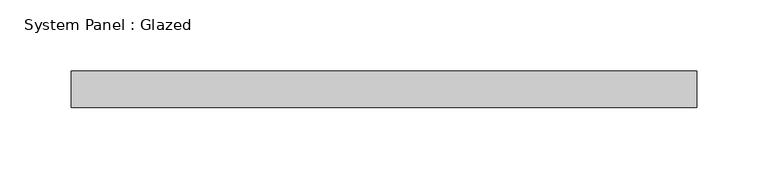
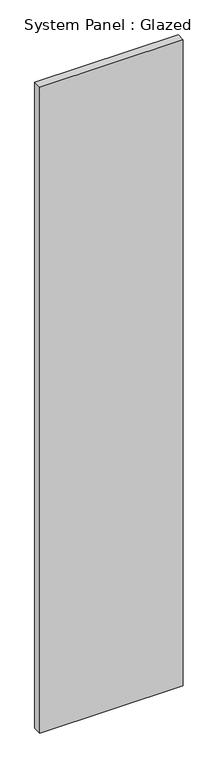
"""IFC4 building model written with IfcOpenShell, lengths in millimetres: plate geometry, System Panel : Glazed."""

from ifc_helpers import new_model, si_unit, origin, origin_with_axes, place, context, project, spatial, polyline, outline, extrude, source, transform, mapped, element, save


def system_panel_glazed_1118b51c(model_context):
    return source(origin(), model_context, "Body", "SweptSolid", [
        extrude(outline(polyline([(219.075, -44.45), (-219.075, -44.45), (-219.075, -19.05), (219.075, -19.05), (219.075, -44.45)])), origin_with_axes(), (0.0, 0.0, 1.0), 2082.8),
    ])


if __name__ == "__main__":
    model = new_model("IFC4")
    model_context = context("Model", 3, world=origin())
    ifc_project = project(units=[si_unit("LENGTHUNIT", "METRE", prefix="MILLI")], contexts=[model_context])
    site = spatial("IfcSite", under=ifc_project)
    building = spatial("IfcBuilding", under=site)
    placement = place(None, origin())
    system_panel_glazed_shape = system_panel_glazed_1118b51c(model_context)
    element("IfcPlate", 1, ObjectType="System Panel : Glazed", at=placement, inside=building, context=model_context, shape_type="MappedRepresentation", body=[
        mapped(system_panel_glazed_shape, transform((0.0, 0.0, 0.0), x_axis=(1.0, 0.0, 0.0), y_axis=(0.0, 1.0, 0.0), z_axis=(0.0, 0.0, 1.0))),
    ])
    save(model, "model.ifc")

# Revit data of these elements
# Type "System Panel : Glazed"
#   Construction Type Id = "GSP4R"
#   Analytic Construction = "1/8 in Pilkington single glazing"
#   Visual Light Transmittance = 0.9
#   Solar Heat Gain Coefficient = 0.86
#   Heat Transfer Coefficient (U) = 1.18115 BTU/(h·ft²·°F)
#   Define Thermal Properties by = 1
# Element 1 (IfcPlate, "System Panel : Glazed")
#   Materials on its faces: "Glass"
# Materials
#   "Glass": class "Glass", colour RGB 0 128 192, transparency 0.75, Description = "Soda Lime Glass", Cost = 0
